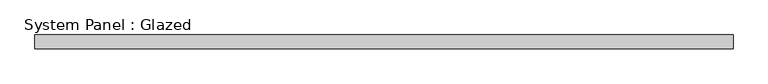
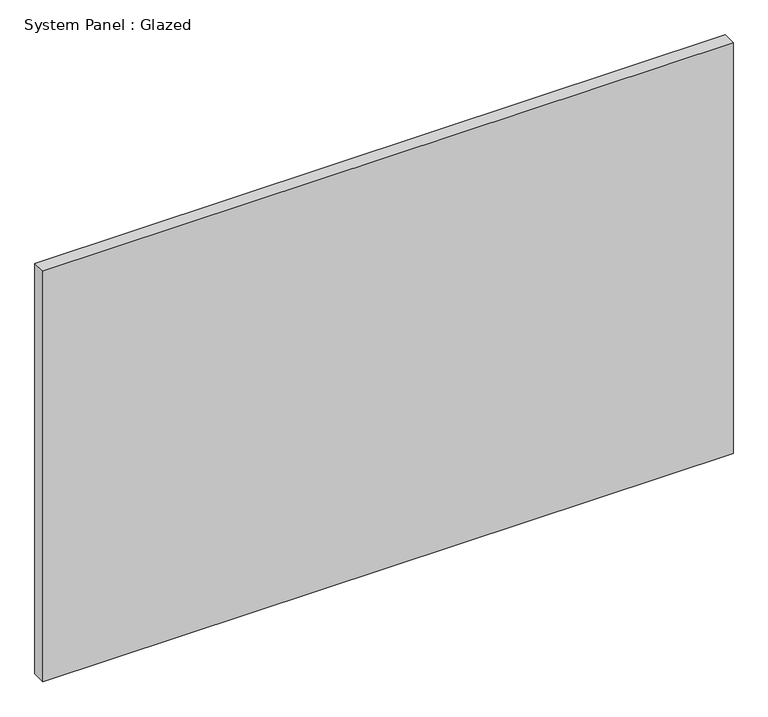
"""IFC4 building model written with IfcOpenShell, lengths in millimetres: plate geometry, System Panel : Glazed."""

from ifc_helpers import new_model, si_unit, origin, origin_with_axes, place, context, project, spatial, polyline, outline, extrude, source, transform, mapped, element, save


def system_panel_glazed_c9ee7fb0(model_context):
    return source(origin(), model_context, "Body", "SweptSolid", [
        extrude(outline(polyline([(650.875, 19.05), (-650.875, 19.05), (-650.875, 44.45), (650.875, 44.45), (650.875, 19.05)])), origin_with_axes(), (0.0, 0.0, 1.0), 819.15),
    ])


if __name__ == "__main__":
    model = new_model("IFC4")
    model_context = context("Model", 3, world=origin())
    ifc_project = project(units=[si_unit("LENGTHUNIT", "METRE", prefix="MILLI")], contexts=[model_context])
    site = spatial("IfcSite", under=ifc_project)
    building = spatial("IfcBuilding", under=site)
    placement = place(None, origin())
    system_panel_glazed_shape = system_panel_glazed_c9ee7fb0(model_context)
    element("IfcPlate", 1, ObjectType="System Panel : Glazed", at=placement, inside=building, context=model_context, shape_type="MappedRepresentation", body=[
        mapped(system_panel_glazed_shape, transform((0.0, 0.0, 0.0), x_axis=(1.0, 0.0, 0.0), y_axis=(0.0, 1.0, 0.0), z_axis=(0.0, 0.0, 1.0))),
    ])
    save(model, "model.ifc")

# Revit data of these elements
# Type "System Panel : Glazed"
#   Construction Type Id = "GSP4R"
#   Analytic Construction = "1/8 in Pilkington single glazing"
#   Visual Light Transmittance = 0.9
#   Solar Heat Gain Coefficient = 0.86
#   Heat Transfer Coefficient (U) = 1.18115 BTU/(h·ft²·°F)
# Element 1 (IfcPlate, "System Panel : Glazed")
#   Materials on its faces: "Glass"
# Materials
#   "Glass": class "Glass", colour RGB 0 128 192, transparency 0.75, Description = "Soda Lime Glass", Cost = 0
